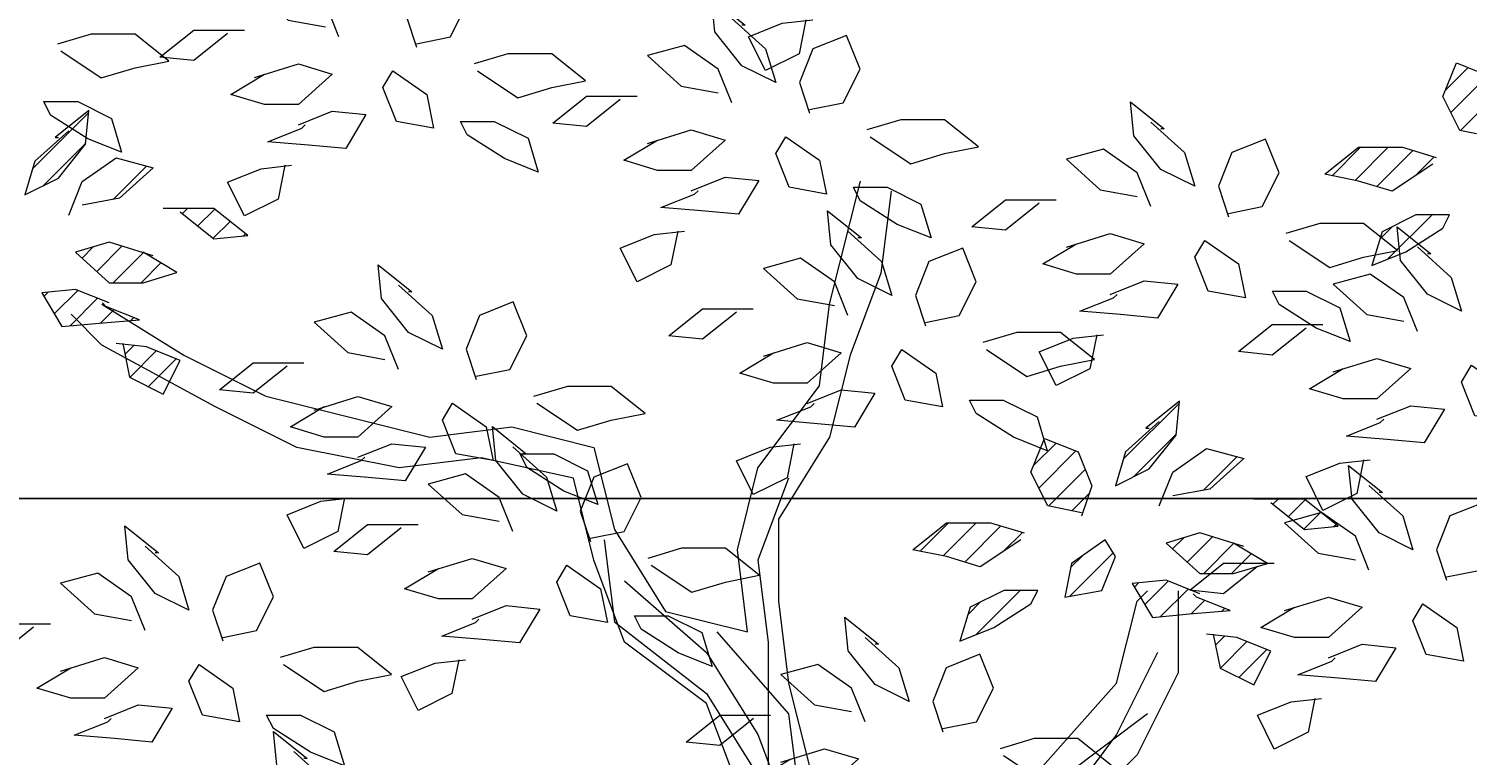
# Model space of a CAD drawing. Units: inches. Extents: x 1770 to 2988, y 1161 to 3221.
# Tile 41 of 44: x 2687 to 2745, y 2796 to 2825. Entities that reach past the tile are written whole.
import ezdxf

# ---------------------------------------------------------------- set-up
doc = ezdxf.new("R2010")
doc.units = ezdxf.units.IN
doc.layers.add('A-ANNO-DIMS', color=2, linetype='Continuous', lineweight=18)
doc.layers.add('trees1', color=250, linetype='Continuous', lineweight=13)
doc.styles.get("Standard").update_dxf_attribs({"font": 'arial.ttf'})
doc.dimstyles.get("Standard").update_dxf_attribs({"dimtxt": 0.18, "dimasz": 0.18, "dimexe": 0.18, "dimexo": 0.0625, "dimgap": 0.09, "dimtad": 0, "dimtih": 1, "dimtoh": 1, "dimdec": 4, "dimzin": 0, "dimdsep": 46, "dimtxsty": 'Standard', "dimcen": 0.09, "dimadec": 0, "dimazin": 0, "dimtfac": 1, "dimtdec": 4, "dimtofl": 0, "dimtmove": 0, "dimatfit": 3, "dimfxl": 1, "dimtolj": 1, "dimtzin": 0, "dimarcsym": 0})

# ---------------------------------------------------------------- blocks, each defined once
blk = doc.blocks.new('*X7')
at = {"color": 0}
for p, q in [((0.66425, -0.90907), (0.66992, -0.90339)), ((0.66732, -0.92367), (0.68419, -0.9068)), ((0.67911, -0.92956), (0.69682, -0.91184))]:
    blk.add_line(p, q, dxfattribs=at)
blk = doc.blocks.new('*X9')
at = {"color": 0}
for p, q in [((0.70074, -0.81954), (0.70399, -0.81629)), ((0.71057, -0.82739), (0.7213, -0.81666)), ((0.72039, -0.83525), (0.73112, -0.82451)), ((0.73958, -0.83373), (0.74095, -0.83237))]:
    blk.add_line(p, q, dxfattribs=at)
blk = doc.blocks.new('*X15')
at = {"color": 0}
for p, q in [((0.60562, -0.79091), (0.64126, -0.75528)), ((0.61243, -0.80179), (0.63929, -0.77492))]:
    blk.add_line(p, q, dxfattribs=at)
blk = doc.blocks.new('*X14')
at = {"color": 0}
blk.add_line((0.65666, -0.81059), (0.67788, -0.78936), dxfattribs=at)
blk = doc.blocks.new('*X6')
at = {"color": 0}
for p, q in [((0.61933, -0.88328), (0.63423, -0.86837)), ((0.61269, -0.87223), (0.61539, -0.86953)), ((0.62935, -0.89093), (0.64686, -0.87342)), ((0.64878, -0.88917), (0.65735, -0.88061)), ((0.66807, -0.88757), (0.66997, -0.88566))]:
    blk.add_line(p, q, dxfattribs=at)
blk = doc.blocks.new('*X8')
at = {"color": 0}
for p, q in [((0.63698, -0.84795), (0.64414, -0.84079)), ((0.64628, -0.85632), (0.66236, -0.84024)), ((0.65678, -0.8635), (0.67596, -0.84432)), ((0.67446, -0.8635), (0.68701, -0.85095))]:
    blk.add_line(p, q, dxfattribs=at)
blk = doc.blocks.new('*X11')
at = {"color": 0}
for p, q in [((0.57164, -0.87793), (0.59916, -0.85041)), ((0.57212, -0.85977), (0.57987, -0.85203))]:
    blk.add_line(p, q, dxfattribs=at)
blk = doc.blocks.new('*X10')
at = {"color": 0}
for p, q in [((0.51178, -0.90243), (0.53998, -0.87423)), ((0.50681, -0.88973), (0.5149, -0.88163))]:
    blk.add_line(p, q, dxfattribs=at)
blk = doc.blocks.new('*X12')
at = {"color": 0}
for p, q in [((0.47641, -0.84941), (0.49451, -0.83131)), ((0.49114, -0.85236), (0.51219, -0.83131)), ((0.5049, -0.85628), (0.52785, -0.83333)), ((0.52956, -0.8493), (0.54145, -0.83741))]:
    blk.add_line(p, q, dxfattribs=at)
blk = doc.blocks.new('*X13')
at = {"color": 0}
for p, q in [((0.54857, -0.79493), (0.56288, -0.78062)), ((0.55195, -0.80923), (0.57551, -0.78567)), ((0.55817, -0.82069), (0.58143, -0.79742)), ((0.5729, -0.82363), (0.58391, -0.81263))]:
    blk.add_line(p, q, dxfattribs=at)
blk = doc.blocks.new('tree342')
at = {"color": 0}
for p, q in [((13.03, 1686.58), (19.55, 1712.62)), ((39.1, 1706.11), (32.58, 1654.02)), ((0, 1634.48), (13.03, 1686.58)), ((32.58, 1654.02), (13.03, 1601.92)), ((-462.65, 1608.43), (-482.2, 1627.97)), ((-462.65, 1634.48), (-410.52, 1601.92)), ((-6.52, 1582.39), (0, 1634.48)), ((-390.97, 1569.36), (-462.65, 1608.43)), ((-410.52, 1601.92), (-358.39, 1575.87)), ((13.03, 1601.92), (0, 1549.83)), ((-45.61, 1530.29), (-6.52, 1582.39)), ((-358.39, 1575.87), (-254.13, 1549.83)), ((-338.84, 1543.32), (-390.97, 1569.36)), ((-254.13, 1549.83), (-202, 1556.34)), ((-202, 1556.34), (-149.87, 1543.32)), ((0, 1549.83), (-32.58, 1497.73)), ((-273.68, 1530.29), (-338.84, 1543.32)), ((-221.55, 1536.8), (-273.68, 1530.29)), ((-162.91, 1523.78), (-221.55, 1536.8)), ((-149.87, 1543.32), (-136.84, 1491.22)), ((-58.65, 1478.2), (-45.61, 1530.29)), ((-149.87, 1471.68), (-162.91, 1523.78)), ((-26.06, 1523.78), (-45.61, 1471.68)), ((-136.84, 1491.22), (-104.26, 1439.13)), ((-32.58, 1497.73), (-32.58, 1445.64)), ((-143.36, 1484.71), (-136.84, 1432.61)), ((-52.13, 1426.1), (-58.65, 1478.2)), ((-130.32, 1419.59), (-149.87, 1471.68)), ((-45.61, 1471.68), (-39.1, 1419.59)), ((-130.32, 1458.66), (-78.19, 1413.08)), ((-32.58, 1445.64), (-26.06, 1393.54)), ((182.45, 1393.54), (195.49, 1445.64)), ((195.49, 1445.64), (202, 1452.15)), ((221.55, 1452.15), (221.55, 1400.05)), ((-104.26, 1439.13), (-52.13, 1426.1)), ((-136.84, 1432.61), (-78.19, 1387.03)), ((-78.19, 1380.52), (-130.32, 1419.59)), ((-71.68, 1426.1), (-26.06, 1374.01)), ((-39.1, 1419.59), (-39.1, 1315.4)), ((-78.19, 1413.08), (-45.61, 1360.98)), ((208.52, 1413.08), (182.45, 1360.98)), ((221.55, 1400.05), (195.49, 1347.96)), ((-26.06, 1393.54), (-13.03, 1341.45)), ((130.32, 1334.94), (182.45, 1393.54)), ((-78.19, 1387.03), (-45.61, 1334.94)), ((-58.65, 1328.42), (-78.19, 1380.52)), ((-26.06, 1374.01), (-19.55, 1321.91)), ((202, 1374.01), (149.87, 1334.94)), ((-45.61, 1360.98), (-26.06, 1308.89)), ((182.45, 1360.98), (143.36, 1308.89)), ((195.49, 1347.96), (143.36, 1295.86))]:
    blk.add_line(p, q, dxfattribs=at)
for points in [[(-311.97, 1804.17), (-320.56, 1825.63), (-342.03, 1840.65), (-365.66, 1834.21), (-344.18, 1814.9), (-320.56, 1810.6)], [(-262.58, 1799.87), (-241.1, 1804.17), (-230.37, 1825.63), (-238.96, 1847.09), (-260.43, 1838.5), (-269.02, 1817.04), (-262.58, 1797.73)], [(-62.2, 1815.93), (-40.73, 1796.62), (-34.29, 1775.16), (-55.76, 1785.89), (-72.94, 1807.35), (-75.09, 1828.81), (-53.61, 1811.64), (-55.76, 1811.64)], [(-15.07, 1815), (-19.37, 1793.54), (-40.84, 1782.81), (-51.58, 1804.27), (-30.1, 1812.85), (-10.78, 1815)], [(-488.8, 1795.28), (-463.03, 1778.11), (-441.55, 1784.55), (-420.08, 1788.84), (-441.55, 1806.01), (-469.47, 1806.01), (-490.95, 1799.57)], [(-382.84, 1806.31), (-404.31, 1789.14), (-425.78, 1791.29), (-404.31, 1808.46), (-372.1, 1808.46)], [(-12.81, 1757.99), (8.66, 1762.28), (19.4, 1783.74), (10.81, 1805.2), (-10.67, 1796.62), (-19.25, 1775.16), (-12.81, 1755.85)], [(-223.92, 1782.71), (-198.16, 1765.54), (-176.68, 1771.98), (-155.21, 1776.27), (-176.68, 1793.44), (-204.6, 1793.44), (-226.07, 1787)], [(-62.2, 1762.28), (-70.79, 1783.74), (-92.27, 1798.77), (-115.89, 1792.33), (-94.42, 1773.01), (-70.79, 1768.72)], [(-365.66, 1778.41), (-337.74, 1787), (-316.26, 1780.56), (-337.74, 1761.25), (-359.21, 1761.25), (-380.69, 1767.68), (-359.21, 1780.56)], [(422.1, 1740.53), (400.62, 1744.82), (389.89, 1766.28), (398.48, 1787.74), (419.95, 1779.15), (428.54, 1757.69), (422.1, 1738.38)], [(-133.07, 1764.43), (-154.54, 1747.26), (-176.02, 1749.41), (-154.54, 1766.58), (-122.33, 1766.58)], [(-483.76, 1744.58), (-505.24, 1725.26), (-511.68, 1703.8), (-490.2, 1714.53), (-473.03, 1735.99), (-470.88, 1757.45), (-492.35, 1740.29), (-490.2, 1740.29)], [(-337.74, 1748.37), (-316.26, 1756.95), (-294.79, 1754.81), (-307.68, 1733.35), (-331.3, 1735.49), (-357.07, 1737.64), (-335.59, 1746.22), (-333.44, 1748.37)], [(204.17, 1750.04), (225.65, 1730.72), (232.09, 1709.26), (210.62, 1719.99), (193.44, 1741.45), (191.29, 1762.91), (212.76, 1745.75), (210.62, 1745.75)], [(25.84, 1740.82), (51.61, 1723.66), (73.09, 1730.09), (94.56, 1734.39), (73.09, 1751.55), (45.17, 1751.55), (23.69, 1745.12)], [(-115.89, 1736.53), (-87.97, 1745.12), (-66.5, 1738.68), (-87.97, 1719.36), (-109.45, 1719.36), (-130.92, 1725.8), (-109.45, 1738.68)], [(253.56, 1692.1), (275.04, 1696.39), (285.78, 1717.85), (277.19, 1739.31), (255.71, 1730.72), (247.12, 1709.26), (253.56, 1689.95)], [(204.17, 1696.39), (195.58, 1717.85), (174.11, 1732.87), (150.49, 1726.43), (171.96, 1707.12), (195.58, 1702.83)], [(383.44, 1723.36), (357.67, 1706.19), (336.2, 1712.63), (314.73, 1716.92), (336.2, 1734.09), (364.12, 1734.09), (385.59, 1727.65)], [(-483.76, 1690.93), (-475.17, 1712.39), (-453.7, 1727.41), (-430.08, 1720.97), (-451.55, 1701.66), (-475.17, 1697.37)], [(-346.33, 1722.62), (-350.62, 1701.16), (-372.1, 1690.43), (-382.84, 1711.89), (-361.36, 1720.47), (-342.03, 1722.62)], [(-87.97, 1706.49), (-66.5, 1715.07), (-45.02, 1712.93), (-57.91, 1691.47), (-81.53, 1693.61), (-107.3, 1695.76), (-85.83, 1704.34), (-83.68, 1706.49)], [(-412.9, 1693.07), (-391.42, 1675.91), (-369.95, 1678.05), (-391.42, 1695.22), (-423.63, 1695.22)], [(11.58, 1680.75), (33.06, 1661.44), (39.5, 1639.98), (18.03, 1650.71), (0.85, 1672.17), (-1.3, 1693.63), (20.17, 1676.46), (18.03, 1676.46)], [(133.31, 1698.53), (111.83, 1681.37), (90.36, 1683.51), (111.83, 1700.68), (144.05, 1700.68)], [(292.22, 1674.93), (317.99, 1657.76), (339.46, 1664.2), (360.94, 1668.49), (339.46, 1685.66), (311.55, 1685.66), (290.07, 1679.22)], [(373.73, 1670.72), (395.2, 1651.41), (401.64, 1629.95), (380.17, 1640.68), (362.99, 1662.14), (360.84, 1683.6), (382.32, 1666.43), (380.17, 1666.43)], [(-430.08, 1665.18), (-457.99, 1673.76), (-479.47, 1667.32), (-457.99, 1648.01), (-436.52, 1648.01), (-415.04, 1654.45), (-436.52, 1667.32)], [(-96.56, 1680.74), (-100.86, 1659.27), (-122.33, 1648.54), (-133.07, 1670.01), (-111.59, 1678.59), (-92.27, 1680.74)], [(150.49, 1670.64), (178.4, 1679.22), (199.88, 1672.78), (178.4, 1653.47), (156.93, 1653.47), (135.46, 1659.91), (156.93, 1672.78)], [(60.97, 1622.81), (82.45, 1627.1), (93.19, 1648.56), (84.6, 1670.02), (63.12, 1661.44), (54.53, 1639.98), (60.97, 1620.66)], [(-274.11, 1646.52), (-252.64, 1627.21), (-246.2, 1605.75), (-267.67, 1616.48), (-284.85, 1637.94), (-287, 1659.4), (-265.52, 1642.23), (-267.67, 1642.23)], [(11.58, 1627.1), (2.99, 1648.56), (-18.48, 1663.58), (-42.1, 1657.15), (-20.63, 1637.83), (2.99, 1633.54)], [(178.4, 1640.59), (199.88, 1649.18), (221.35, 1647.03), (208.47, 1625.57), (184.85, 1627.72), (159.08, 1629.86), (180.55, 1638.45), (182.7, 1640.59)], [(373.73, 1617.07), (365.14, 1638.53), (343.66, 1653.55), (320.04, 1647.12), (341.51, 1627.8), (365.14, 1623.51)], [(-457.99, 1635.13), (-479.47, 1643.72), (-500.94, 1641.57), (-488.06, 1620.11), (-464.44, 1622.26), (-438.67, 1624.4), (-460.14, 1632.99), (-462.29, 1635.13)], [(-274.11, 1592.87), (-282.7, 1614.33), (-304.18, 1629.35), (-327.8, 1622.91), (-306.33, 1603.6), (-282.7, 1599.31)], [(-224.72, 1588.58), (-203.25, 1592.87), (-192.51, 1614.33), (-201.1, 1635.79), (-222.58, 1627.21), (-231.17, 1605.75), (-224.72, 1586.43)], [(-59.28, 1629.25), (-80.76, 1612.08), (-102.23, 1614.22), (-80.76, 1631.39), (-48.55, 1631.39)], [(302.86, 1619.22), (281.39, 1602.05), (259.91, 1604.2), (281.39, 1621.36), (313.6, 1621.36)], [(-42.1, 1601.35), (-14.19, 1609.93), (7.29, 1603.49), (-14.19, 1584.18), (-35.66, 1584.18), (-57.14, 1590.62), (-35.66, 1603.49)], [(99.63, 1605.64), (125.4, 1588.47), (146.87, 1594.91), (168.35, 1599.2), (146.87, 1616.37), (118.96, 1616.37), (97.48, 1609.93)], [(169.81, 1614.84), (165.52, 1593.38), (144.05, 1582.65), (133.31, 1604.11), (154.78, 1612.69), (174.11, 1614.84)], [(-449.4, 1609.38), (-445.11, 1587.92), (-423.63, 1577.19), (-412.9, 1598.65), (-434.37, 1607.23), (-453.7, 1609.38)], [(-344.98, 1595.02), (-366.45, 1577.85), (-387.93, 1579.99), (-366.45, 1597.16), (-334.24, 1597.16)], [(320.04, 1591.32), (347.96, 1599.9), (369.43, 1593.47), (347.96, 1574.15), (326.48, 1574.15), (305.01, 1580.59), (326.48, 1593.47)], [(-186.07, 1571.41), (-160.3, 1554.24), (-138.83, 1560.68), (-117.35, 1564.97), (-138.83, 1582.14), (-166.74, 1582.14), (-188.22, 1575.7)], [(-327.8, 1567.12), (-299.88, 1575.7), (-278.41, 1569.26), (-299.88, 1549.95), (-321.36, 1549.95), (-342.83, 1556.39), (-321.36, 1569.26)], [(-14.19, 1571.3), (7.29, 1579.89), (28.76, 1577.74), (15.88, 1556.28), (-7.74, 1558.43), (-33.51, 1560.57), (-12.04, 1569.16), (-9.89, 1571.3)], [(209.56, 1559.81), (188.09, 1540.5), (181.65, 1519.04), (203.12, 1529.77), (220.3, 1551.23), (222.45, 1572.69), (200.98, 1555.52), (203.12, 1555.52)], [(347.96, 1561.28), (369.43, 1569.86), (390.91, 1567.71), (378.02, 1546.25), (354.4, 1548.4), (328.63, 1550.55), (350.1, 1559.13), (352.25, 1561.28)], [(-201.46, 1543.66), (-179.98, 1524.35), (-173.54, 1502.89), (-195.02, 1513.62), (-212.2, 1535.08), (-214.34, 1556.54), (-192.87, 1539.37), (-195.02, 1539.37)], [(-299.88, 1537.07), (-278.41, 1545.66), (-256.93, 1543.51), (-269.82, 1522.05), (-293.44, 1524.2), (-319.21, 1526.34), (-297.74, 1534.93), (-295.59, 1537.07)], [(-22.78, 1545.55), (-27.07, 1524.09), (-48.55, 1513.36), (-59.28, 1534.82), (-37.81, 1543.41), (-18.48, 1545.55)], [(160.17, 1501.87), (138.7, 1506.16), (127.96, 1527.62), (136.55, 1549.08), (158.03, 1540.5), (166.62, 1519.04), (160.17, 1499.73)], [(209.56, 1506.16), (218.15, 1527.62), (239.63, 1542.65), (263.25, 1536.21), (241.78, 1516.89), (218.15, 1512.6)], [(-152.07, 1485.72), (-130.59, 1490.01), (-119.86, 1511.47), (-128.45, 1532.93), (-149.92, 1524.35), (-158.51, 1502.89), (-152.07, 1483.57)], [(339.37, 1535.52), (335.07, 1514.06), (313.6, 1503.33), (302.86, 1524.79), (324.33, 1533.38), (343.66, 1535.52)], [(342.84, 1519.08), (364.31, 1499.77), (370.76, 1478.31), (349.28, 1489.04), (332.1, 1510.5), (329.95, 1531.96), (351.43, 1514.79), (349.28, 1514.79)], [(-201.46, 1490.01), (-210.05, 1511.47), (-231.52, 1526.49), (-255.15, 1520.05), (-233.67, 1500.74), (-210.05, 1496.45)], [(-308.47, 1511.32), (-312.77, 1489.86), (-334.24, 1479.13), (-344.98, 1500.59), (-323.51, 1509.18), (-304.18, 1511.32)], [(280.43, 1508.31), (301.91, 1491.14), (323.38, 1493.29), (301.91, 1510.46), (269.69, 1510.46)], [(342.84, 1465.43), (334.25, 1486.89), (312.78, 1501.91), (289.15, 1495.48), (310.63, 1476.16), (334.25, 1471.87)], [(392.23, 1461.14), (413.7, 1465.43), (424.44, 1486.89), (415.85, 1508.35), (394.38, 1499.77), (385.79, 1478.31), (392.23, 1458.99)], [(-435.23, 1480.59), (-413.75, 1461.28), (-407.31, 1439.82), (-428.79, 1450.55), (-445.97, 1472.01), (-448.11, 1493.47), (-426.64, 1476.3), (-428.79, 1476.3)], [(-272.32, 1492.16), (-293.8, 1474.99), (-315.27, 1477.13), (-293.8, 1494.3), (-261.59, 1494.3)], [(121.52, 1484.7), (95.75, 1467.54), (74.28, 1473.97), (52.8, 1478.27), (74.28, 1495.43), (102.19, 1495.43), (123.67, 1489)], [(263.25, 1480.41), (235.33, 1489), (213.86, 1482.56), (235.33, 1463.24), (256.81, 1463.24), (278.28, 1469.68), (256.81, 1482.56)], [(-255.15, 1464.26), (-227.23, 1472.84), (-205.75, 1466.4), (-227.23, 1447.09), (-248.7, 1447.09), (-270.18, 1453.53), (-248.7, 1466.4)], [(-113.41, 1468.55), (-87.64, 1451.38), (-66.17, 1457.82), (-44.7, 1462.11), (-66.17, 1479.28), (-94.09, 1479.28), (-115.56, 1472.84)], [(-435.23, 1426.94), (-443.82, 1448.4), (-465.29, 1463.42), (-488.91, 1456.98), (-467.44, 1437.67), (-443.82, 1433.38)], [(-385.84, 1422.65), (-364.36, 1426.94), (-353.63, 1448.4), (-362.22, 1469.86), (-383.69, 1461.28), (-392.28, 1439.82), (-385.84, 1420.5)], [(271.97, 1467.58), (250.5, 1450.41), (229.02, 1452.56), (250.5, 1469.72), (282.71, 1469.72)], [(235.33, 1450.37), (213.86, 1458.95), (192.39, 1456.81), (205.27, 1435.35), (228.89, 1437.49), (254.66, 1439.64), (233.19, 1448.22), (231.04, 1450.37)], [(289.15, 1439.68), (317.07, 1448.26), (338.54, 1441.83), (317.07, 1422.51), (295.6, 1422.51), (274.12, 1428.95), (295.6, 1441.83)], [(-227.23, 1434.21), (-205.75, 1442.8), (-184.28, 1440.65), (-197.16, 1419.19), (-220.79, 1421.34), (-246.56, 1423.48), (-225.08, 1432.07), (-222.93, 1434.21)], [(-506.09, 1429.09), (-527.57, 1411.92), (-549.04, 1414.06), (-527.57, 1431.23), (-495.36, 1431.23)], [(22.56, 1422.65), (44.03, 1403.34), (50.48, 1381.88), (29, 1392.61), (11.82, 1414.07), (9.68, 1435.53), (31.15, 1418.36), (29, 1418.36)], [(243.92, 1424.62), (248.22, 1403.16), (269.69, 1392.43), (280.43, 1413.89), (258.96, 1422.47), (239.63, 1424.62)], [(317.07, 1409.64), (338.54, 1418.22), (360.02, 1416.07), (347.13, 1394.61), (323.51, 1396.76), (297.74, 1398.91), (319.22, 1407.49), (321.36, 1409.64)], [(-488.91, 1401.19), (-461, 1409.77), (-439.52, 1403.33), (-461, 1384.02), (-482.47, 1384.02), (-503.95, 1390.46), (-482.47, 1403.33)], [(-347.18, 1405.48), (-321.41, 1388.31), (-299.94, 1394.75), (-278.46, 1399.04), (-299.94, 1416.21), (-327.86, 1416.21), (-349.33, 1409.77)], [(-235.82, 1408.46), (-240.11, 1387), (-261.59, 1376.27), (-272.32, 1397.73), (-250.85, 1406.32), (-231.52, 1408.46)], [(71.95, 1364.71), (93.43, 1369), (104.16, 1390.46), (95.57, 1411.92), (74.1, 1403.34), (65.51, 1381.88), (71.95, 1362.56)], [(22.56, 1369), (13.97, 1390.46), (-7.5, 1405.48), (-31.13, 1399.05), (-9.65, 1379.73), (13.97, 1375.44)], [(308.48, 1383.88), (304.19, 1362.42), (282.71, 1351.69), (271.97, 1373.15), (293.45, 1381.74), (312.78, 1383.88)], [(-461, 1371.14), (-439.52, 1379.73), (-418.05, 1377.58), (-430.93, 1356.12), (-454.56, 1358.27), (-480.32, 1360.41), (-458.85, 1369), (-456.7, 1371.14)], [(-48.31, 1371.15), (-69.78, 1353.98), (-91.25, 1356.12), (-69.78, 1373.29), (-37.57, 1373.29)], [(-340.71, 1350.05), (-319.24, 1330.73), (-312.8, 1309.27), (-334.27, 1320), (-351.45, 1341.46), (-353.6, 1362.92), (-332.12, 1345.75), (-334.27, 1345.75)], [(110.61, 1347.54), (136.38, 1330.37), (157.85, 1336.81), (179.32, 1341.1), (157.85, 1358.27), (129.93, 1358.27), (108.46, 1351.83)], [(-31.13, 1343.25), (-3.21, 1351.83), (18.27, 1345.39), (-3.21, 1326.08), (-24.68, 1326.08), (-46.16, 1332.52), (-24.68, 1345.39)]]:
    blk.add_lwpolyline(points, dxfattribs=at)
for points in [[(-256.14, 1767.68), (-251.84, 1746.22), (-275.46, 1750.52), (-284.05, 1771.98), (-277.61, 1782.71)], [(-478.06, 1763.09), (-456.59, 1752.36), (-450.14, 1730.9), (-471.62, 1739.48), (-495.24, 1754.5), (-499.54, 1763.09)], [(-213.19, 1750.52), (-191.71, 1739.79), (-185.27, 1718.33), (-206.75, 1726.91), (-230.37, 1741.93), (-234.66, 1750.52)], [(-6.37, 1725.8), (-2.08, 1704.34), (-25.7, 1708.63), (-34.29, 1730.09), (-27.84, 1740.82)], [(36.58, 1708.63), (58.05, 1697.9), (64.5, 1676.44), (43.02, 1685.03), (19.4, 1700.05), (15.1, 1708.63)], [(372.71, 1691.17), (351.23, 1680.44), (344.79, 1658.98), (366.26, 1667.56), (389.89, 1682.58), (394.18, 1691.17)], [(260.01, 1659.91), (264.3, 1638.45), (240.68, 1642.74), (232.09, 1664.2), (238.53, 1674.93)], [(302.96, 1642.74), (324.43, 1632.01), (330.87, 1610.55), (309.4, 1619.13), (285.78, 1634.15), (281.48, 1642.74)], [(67.42, 1590.62), (71.71, 1569.16), (48.09, 1573.45), (39.5, 1594.91), (45.94, 1605.64)], [(429.56, 1580.59), (433.85, 1559.13), (410.23, 1563.42), (401.64, 1584.88), (408.09, 1595.61)], [(110.37, 1573.45), (131.84, 1562.72), (138.28, 1541.26), (116.81, 1549.84), (93.19, 1564.87), (88.89, 1573.45)], [(-218.28, 1556.39), (-213.99, 1534.93), (-237.61, 1539.22), (-246.2, 1560.68), (-239.76, 1571.41)], [(-175.33, 1539.22), (-153.86, 1528.49), (-147.41, 1507.03), (-168.89, 1515.61), (-192.51, 1530.64), (-196.81, 1539.22)], [(153.73, 1469.68), (149.44, 1448.22), (173.06, 1452.51), (181.65, 1473.97), (175.21, 1484.7)], [(-145.63, 1453.53), (-141.33, 1432.07), (-164.95, 1436.36), (-173.54, 1457.82), (-167.1, 1468.55)], [(110.78, 1452.51), (89.31, 1441.78), (82.87, 1420.32), (104.34, 1428.91), (127.96, 1443.93), (132.26, 1452.51)], [(-102.68, 1436.36), (-81.2, 1425.63), (-74.76, 1404.17), (-96.23, 1412.75), (-119.86, 1427.78), (-124.15, 1436.36)], [(398.67, 1428.95), (402.97, 1407.49), (379.35, 1411.78), (370.76, 1433.24), (377.2, 1443.97)], [(-379.39, 1390.46), (-375.1, 1369), (-398.72, 1373.29), (-407.31, 1394.75), (-400.87, 1405.48)], [(-336.45, 1373.29), (-314.97, 1362.56), (-308.53, 1341.1), (-330, 1349.68), (-353.63, 1364.71), (-357.92, 1373.29)]]:
    blk.add_lwpolyline(points, close=True, dxfattribs=at)
at = {"color": 0, "xscale": 1000, "yscale": 1000, "zscale": 1000}
for name, p in [('*X13', (-157.01, 2565.4)), ('*X15', (-1112.26, 2511.51)), ('*X12', (-157.01, 2565.4)), ('*X14', (-1112.26, 2511.51)), ('*X9', (-1112.26, 2511.51)), ('*X10', (-157.01, 2565.4)), ('*X8', (-1112.26, 2511.51)), ('*X6', (-1112.26, 2511.51)), ('*X7', (-1112.26, 2511.51)), ('*X15', (-418.93, 2326.75)), ('*X13', (-418.93, 2326.75)), ('*X14', (-418.93, 2326.75)), ('*X9', (-418.93, 2326.75)), ('*X12', (-418.93, 2326.75)), ('*X8', (-418.93, 2326.75)), ('*X11', (-418.93, 2326.75)), ('*X6', (-418.93, 2326.75)), ('*X10', (-418.93, 2326.75)), ('*X7', (-418.93, 2326.75))]:
    blk.add_blockref(name, p, dxfattribs=at)
blk = doc.blocks.new('*D97')
at = {"layer": 'A-ANNO-DIMS', "color": 0, "lineweight": -2, "transparency": 16777216}
for p, q in [((2620.113, 2806.297), (2801.915, 2806.297)), ((2801.735, 2806.117), (2801.735, 2782.479)), ((2801.735, 2758.477), (2801.735, 2782.115)), ((2620.113, 2758.297), (2801.915, 2758.297))]:
    blk.add_line(p, q, dxfattribs=at)
at = {"layer": 'A-ANNO-DIMS', "color": 0, "transparency": 16777216}
for points in [[(2801.705, 2806.117), (2801.765, 2806.117), (2801.735, 2806.297)], [(2801.705, 2758.477), (2801.765, 2758.477), (2801.735, 2758.297)]]:
    blk.add_solid(points, dxfattribs=at)
at = {"layer": 'Defpoints', "color": 0, "transparency": 16777216}
for p in [(2620.051, 2806.297), (2801.735, 2806.297), (2620.051, 2758.297)]:
    blk.add_point(p, dxfattribs=at)
at = {"layer": 'A-ANNO-DIMS', "color": 0, "transparency": 16777216, "insert": (2801.735, 2782.297), "char_height": 0.18, "attachment_point": 5}
blk.add_mtext('\\A1;48', dxfattribs=at)
blk = doc.blocks.new('*D98')
at = {"layer": 'A-ANNO-DIMS', "color": 0, "lineweight": -2, "transparency": 16777216}
for p, q in [((2655.505, 2842.297), (2801.915, 2842.297)), ((2801.735, 2842.117), (2801.735, 2824.479)), ((2801.735, 2806.477), (2801.735, 2824.115)), ((2620.113, 2806.297), (2801.915, 2806.297))]:
    blk.add_line(p, q, dxfattribs=at)
at = {"layer": 'A-ANNO-DIMS', "color": 0, "transparency": 16777216}
for points in [[(2801.705, 2842.117), (2801.765, 2842.117), (2801.735, 2842.297)], [(2801.705, 2806.477), (2801.765, 2806.477), (2801.735, 2806.297)]]:
    blk.add_solid(points, dxfattribs=at)
at = {"layer": 'Defpoints', "color": 0, "transparency": 16777216}
for p in [(2655.443, 2842.297), (2801.735, 2842.297), (2620.051, 2806.297)]:
    blk.add_point(p, dxfattribs=at)
at = {"layer": 'A-ANNO-DIMS', "color": 0, "transparency": 16777216, "insert": (2801.735, 2824.297), "char_height": 0.18, "attachment_point": 5}
blk.add_mtext('\\A1;36', dxfattribs=at)

msp = doc.modelspace()

# ---------------------------------------------------------------- block references
at = {"layer": 'trees1', "xscale": 0.063143750371755, "yscale": 0.063143750371755, "zscale": 0.063143750371755}
msp.add_blockref('tree342', (2719.3275, 2710.8976), dxfattribs=at)

# ---------------------------------------------------------------- dimensions: what is measured, and where the dimension line sits
at = {"layer": 'A-ANNO-DIMS'}
for base, p1, p2, picture, middle in [((2801.7346, 2842.2969), (2620.0508, 2806.2969), (2655.443, 2842.2969), '*D98', (2801.7346, 2824.2969)), ((2801.7346, 2806.2969), (2620.0508, 2758.2969), (2620.0508, 2806.2969), '*D97', (2801.7346, 2782.2969))]:
    dim = msp.add_linear_dim(base=base, p1=p1, p2=p2, angle=90, dimstyle='Standard', override={"dimdec": 0, "dimlfac": 1, "dimrnd": 0, "dimzin": 0, "dimdsep": 46, "dimlunit": 2}, dxfattribs=at)
    dim.commit()
    dim.dimension.update_dxf_attribs({"geometry": picture, "text_midpoint": middle})

doc.saveas('drawing.dxf')
